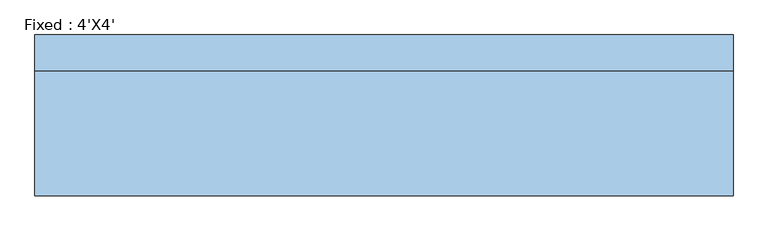
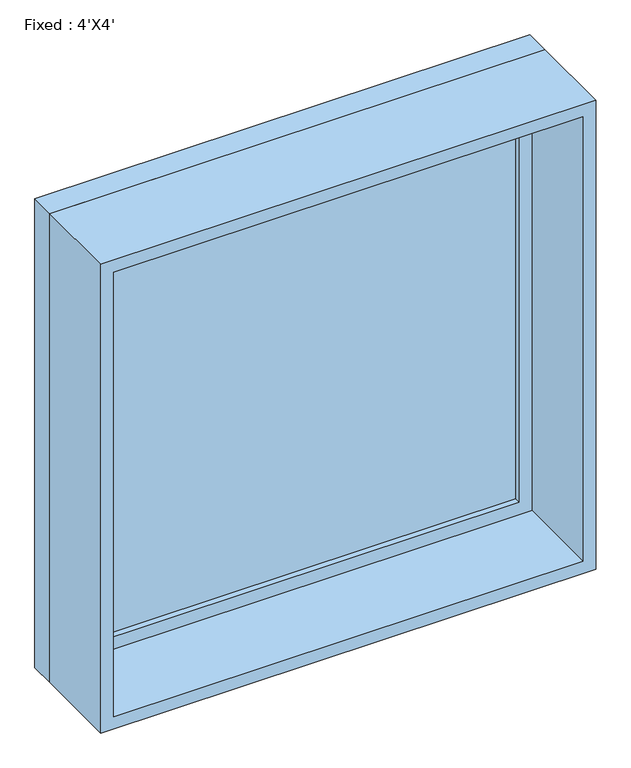
"""IFC4 building model written with IfcOpenShell, lengths in millimetres: window geometry, Fixed : 4'X4'."""

from ifc_helpers import new_model, si_unit, frame, origin, place, context, project, spatial, polyline, outline, extrude, source, transform, mapped, element, save


def fixed_4_x4_67ff7140(model_context):
    return source(origin(), model_context, "Body", "SweptSolid", [
        extrude(outline(polyline([(508.0, 92.775), (-584.2, 92.775), (-584.2, 105.475), (508.0, 105.475), (508.0, 92.775)])), frame((0.0, 0.0, 977.9), z_axis=(0.0, 0.0, 1.0), x_axis=(1.0, 0.0, 0.0)), (0.0, 0.0, 1.0), 1092.2),
        extrude(outline(polyline([(2114.55, -628.65), (933.45, -628.65), (933.45, 552.45), (2114.55, 552.45), (2114.55, -628.65)]), holes=[polyline([(2070.1, -584.2), (2070.1, 508.0), (977.9, 508.0), (977.9, -584.2), (2070.1, -584.2)])]), frame((0.0, 76.9, 0.0), z_axis=(0.0, 1.0, 0.0), x_axis=(0.0, 0.0, 1.0)), (0.0, 0.0, 1.0), 44.45),
        extrude(outline(polyline([(2133.6, -647.7), (914.4, -647.7), (914.4, 571.5), (2133.6, 571.5), (2133.6, -647.7)]), holes=[polyline([(2101.85, -615.95), (2101.85, 539.75), (946.15, 539.75), (946.15, -615.95), (2101.85, -615.95)])]), frame((0.0, -140.4, 0.0), z_axis=(0.0, 1.0, 0.0), x_axis=(0.0, 0.0, 1.0)), (0.0, 0.0, 1.0), 217.3),
        extrude(outline(polyline([(2133.6, 571.5), (2133.6, -647.7), (914.4, -647.7), (914.4, 571.5), (2133.6, 571.5)]), holes=[polyline([(2114.55, 552.45), (933.45, 552.45), (933.45, -628.65), (2114.55, -628.65), (2114.55, 552.45)])]), frame((0.0, 76.9, 0.0), z_axis=(0.0, 1.0, 0.0), x_axis=(0.0, 0.0, 1.0)), (0.0, 0.0, 1.0), 63.5),
    ])


if __name__ == "__main__":
    model = new_model("IFC4")
    model_context = context("Model", 3, world=origin())
    ifc_project = project(units=[si_unit("LENGTHUNIT", "METRE", prefix="MILLI")], contexts=[model_context])
    site = spatial("IfcSite", under=ifc_project)
    building = spatial("IfcBuilding", under=site)
    placement = place(None, origin())
    fixed_4_x4_shape = fixed_4_x4_67ff7140(model_context)
    element("IfcWindow", 1, ObjectType="Fixed : 4'X4'", at=placement, inside=building, context=model_context, shape_type="MappedRepresentation", body=[
        mapped(fixed_4_x4_shape, transform((0.0, 0.0, 0.0), x_axis=(1.0, 0.0, 0.0), y_axis=(0.0, 1.0, 0.0), z_axis=(0.0, 0.0, 1.0))),
    ])
    save(model, "model.ifc")

# Revit data of these elements
# Type "Fixed : 4'X4'"
#   Type Mark = "10"
#   Assembly Code = "B2020100"
#   Height = 4' - 0"
#   Default Sill Height = 3' - 0"
#   Width = 4' - 0"
#   Window Inset = 0' - 0 3/4"
#   Glass Pane Material = Glass
#   Sash Material = Sash
#   Wall Closure = (empty or 0)
# Element 1 (IfcWindow, "Fixed : 4'X4'")
#   Materials on its faces: "Sash", "Glass"
# Materials
#   "Glass": class "Glass", colour RGB 218 227 224, transparency 0.85, Description = "Soda Lime Glass", Cost = 0
#   "Sash": class "Wood", colour RGB 136 99 55, transparency 0
